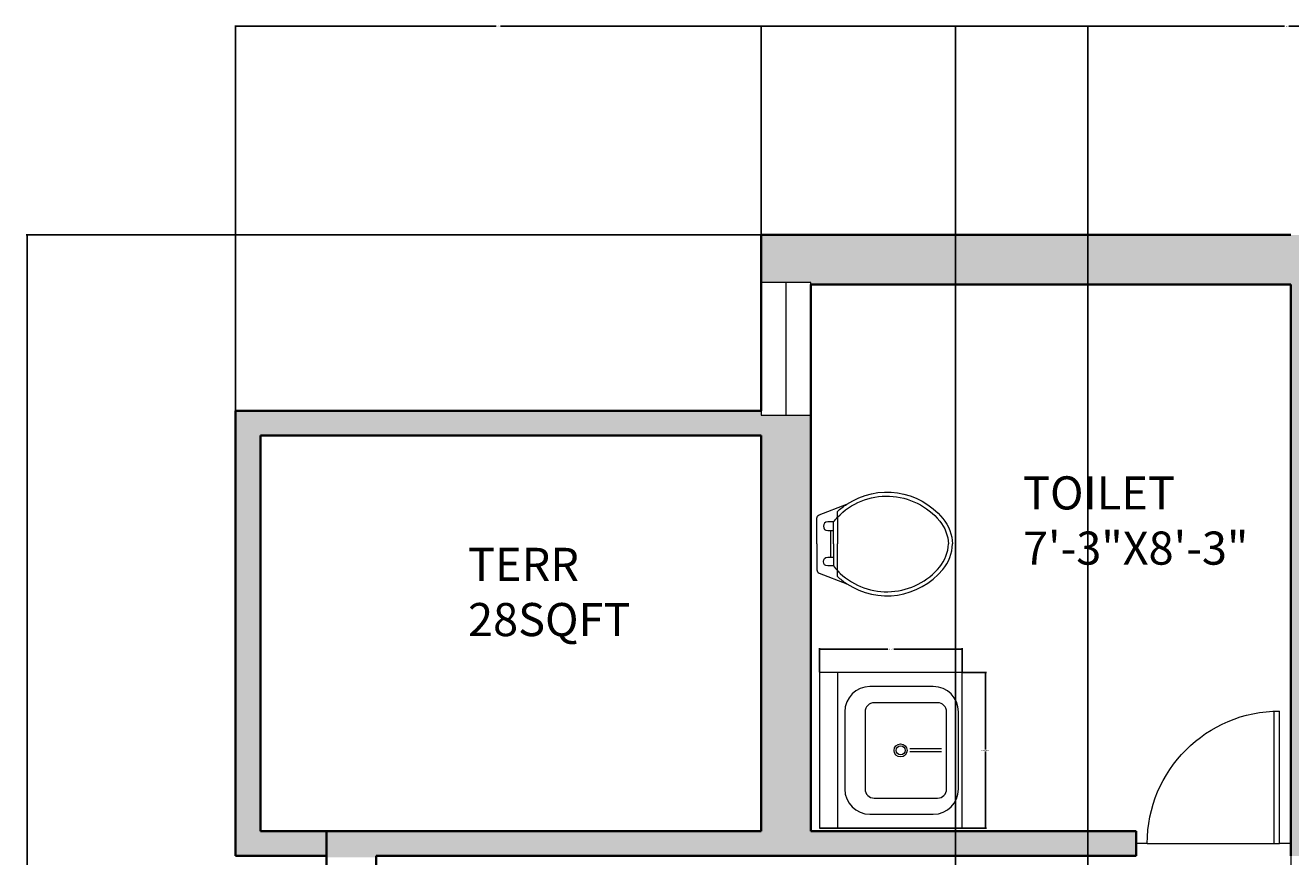
# Model space of a CAD drawing. Units: inches. Extents: x -36 to 442, y -676 to 151.
# Tile 6 of 8: x -36 to 193, y 1 to 151. Entities that reach past the tile are written whole.
import ezdxf

# ---------------------------------------------------------------- set-up
doc = ezdxf.new("R2010")
doc.units = ezdxf.units.IN
doc.header["$MEASUREMENT"] = 0
for name, color, linetype, lineweight in [('A-ANNO-DIMS', 2, 'Continuous', 18), ('A-AREA-IDEN', 7, 'Continuous', 18), ('A-DOOR', 4, 'Continuous', 18), ('A-FLOR-CASE', 32, 'Continuous', 18), ('A-FLOR-FIXT', 9, 'Continuous', 18), ('A-GLAZ', 4, 'Continuous', 13), ('A-WALL', 7, 'Continuous', 35), ('A-WALL-PATT', 8, 'Continuous', 13)]:
    doc.layers.add(name, color=color, linetype=linetype, lineweight=lineweight)
doc.styles.get("Standard").update_dxf_attribs({"font": 'arial.ttf'})
doc.dimstyles.get("Standard").update_dxf_attribs({"dimtxt": 0.18, "dimasz": 0.18, "dimexe": 0.18, "dimexo": 0.0625, "dimgap": 0.09, "dimtad": 0, "dimtih": 1, "dimtoh": 1, "dimdec": 0, "dimzin": 0, "dimdsep": 46, "dimlunit": 3, "dimtxsty": 'Standard', "dimcen": 0.09, "dimadec": 0, "dimazin": 0, "dimtfac": 1, "dimtdec": 0, "dimtofl": 0, "dimtmove": 0, "dimatfit": 3, "dimfxl": 1, "dimtolj": 1, "dimtzin": 0, "dimarcsym": 0})

# ---------------------------------------------------------------- blocks, each defined once
blk = doc.blocks.new('М14 600х655')
for p, q in [((-655, 600), (-655, 0)), ((-655, 600), (-655, 0)), ((-655, 0), (-655, 600)), ((0, 600), (-655, 600)), ((0, 0), (0, 600)), ((0, 525), (-655, 525)), ((-165.1, 494.1), (-489.9, 494.1)), ((-595.8, 388.1), (-595.8, 121.3)), ((-165.4, 408.4), (-490.2, 408.4)), ((-59.2, 121.3), (-59.2, 388.1)), ((-528.4, 370.1), (-528.4, 103.3)), ((-127.2, 103.3), (-127.2, 370.1)), ((-333.5, 87.1), (-333.5, 219.6)), ((-321.5, 87.1), (-321.5, 219.6)), ((-490.2, 65.1), (-165.4, 65.1)), ((-655, 0), (-655, 0)), ((-655, 0), (-655, 0)), ((-655, 0), (0, 0)), ((-655, 0), (0, 0)), ((-489.9, 15.4), (-165.1, 15.4))]:
    blk.add_line(p, q)
for radius in [27.6, 19.3]:
    blk.add_circle((-327.5, 258.9), radius)
for centre, radius, start, end in [((-489.9, 388.1), 105.9, 90, 180), ((-165.1, 388.1), 105.9, 0, 90), ((-490.2, 370.1), 38.2, 90, 180), ((-165.4, 370.1), 38.2, 0, 90), ((-489.9, 121.3), 105.9, 180, 270), ((-165.1, 121.3), 105.9, 270, 0), ((-490.2, 103.3), 38.2, 180, 270), ((-165.4, 103.3), 38.2, 270, 0)]:
    blk.add_arc(centre, radius, start, end)
blk = doc.blocks.new('DOOR-SWING-24IN')
for p, q in [((24, 26), (24, 28)), ((24, 26), (24, 2)), ((24, 3), (0, 3)), ((24, 2), (0, 2)), ((24, 0), (24, 2))]:
    blk.add_line(p, q)
blk.add_arc((24, 2), 24, 90, 180)
blk = doc.blocks.new('WC-PLAN')
for p, q in [((3.72, 14.23), (3.72, 15.26)), ((3.72, 14.23), (3.72, 9.39)), ((3.72, 4.56), (3.72, 9.39)), ((3.72, 3.52), (3.72, 4.56))]:
    blk.add_line(p, q)
for points in [[(5.41, 16.59, -0.383919), (22.82, 14.02, -0.163732), (24.59, 9.39, -0.359733)], [(0, 9.39), (0, 14.09, -0.31031), (0.4, 14.66), (5.41, 16.59, -0.209071)], [(3.72, 14.23, -0.448546), (22.25, 13.55, -0.162618), (23.85, 9.39, -0.470877)], [(3.72, 15.26, -0.040937), (5.41, 16.59, -0.163732)], [(2.98, 13.38, -0.022712), (3.72, 14.23, -0.162618)], [(2.98, 13.38), (1.95, 13.38, 1), (1.95, 11.81), (2.49, 11.81)], [(2.98, 9.39), (2.98, 13.38, -0.476108)], [(0, 9.39), (0, 4.7, 0.31031), (0.4, 4.12), (5.41, 2.19, 0.209071)], [(2.98, 9.39), (2.98, 5.4, 0.022712)], [(4.22, 4.06, 0.431639), (22.25, 5.24, 0.162618), (23.85, 9.39, 0.470877)], [(5.41, 2.19, 0.383919), (22.82, 4.77, 0.163732), (24.59, 9.39, 0.359733)], [(2.98, 5.4), (1.95, 5.4, -1), (1.95, 6.97), (2.49, 6.97)], [(2.98, 5.4, 0.022712), (3.72, 4.56, 0.162618)], [(3.72, 4.56, 0.014165), (4.22, 4.06, 0.162618)], [(3.72, 3.52, 0.040937), (5.41, 2.19, 0.163732)]]:
    blk.add_lwpolyline(points, format="xyb")
for points in [[(2.49, 11.81), (2.49, 6.97)], [(2.49, 11.81), (2.98, 11.81)], [(2.49, 6.97), (2.98, 6.97)]]:
    blk.add_lwpolyline(points)
blk = doc.blocks.new('*D27')
at = {"layer": 'A-ANNO-DIMS', "color": 0, "lineweight": -2, "transparency": 16777216}
for p, q in [((134, 34.23), (138.35, 34.23)), ((138.17, 34.05), (138.17, 20.31)), ((138.17, 6.2), (138.17, 19.94)), ((134, 6.02), (138.35, 6.02))]:
    blk.add_line(p, q, dxfattribs=at)
at = {"layer": 'A-ANNO-DIMS', "color": 0, "transparency": 16777216}
for points in [[(138.14, 34.05), (138.2, 34.05), (138.17, 34.23)], [(138.14, 6.2), (138.2, 6.2), (138.17, 6.02)]]:
    blk.add_solid(points, dxfattribs=at)
at = {"layer": 'Defpoints', "color": 0, "transparency": 16777216}
for p in [(133.94, 34.23), (138.17, 34.23), (133.94, 6.02)]:
    blk.add_point(p, dxfattribs=at)
at = {"layer": 'A-ANNO-DIMS', "color": 0, "transparency": 16777216, "insert": (138.17, 20.12), "char_height": 0.18, "attachment_point": 5}
blk.add_mtext('\\A1;BASIN 28 TYP.', dxfattribs=at)
blk = doc.blocks.new('*D28')
at = {"layer": 'A-ANNO-DIMS', "color": 0, "lineweight": -2, "transparency": 16777216}
for p, q in [((108.1, 34.29), (108.1, 38.64)), ((108.28, 38.46), (120.49, 38.46)), ((133.76, 38.46), (121.55, 38.46)), ((133.94, 34.29), (133.94, 38.64))]:
    blk.add_line(p, q, dxfattribs=at)
at = {"layer": 'A-ANNO-DIMS', "color": 0, "transparency": 16777216}
for points in [[(108.28, 38.49), (108.28, 38.43), (108.1, 38.46)], [(133.76, 38.49), (133.76, 38.43), (133.94, 38.46)]]:
    blk.add_solid(points, dxfattribs=at)
at = {"layer": 'Defpoints', "color": 0, "transparency": 16777216}
for p in [(108.1, 38.46), (108.1, 34.23), (133.94, 34.23)]:
    blk.add_point(p, dxfattribs=at)
at = {"layer": 'A-ANNO-DIMS', "color": 0, "transparency": 16777216, "insert": (121.02, 38.46), "char_height": 0.18, "attachment_point": 5}
blk.add_mtext('\\A1;26 TYP.', dxfattribs=at)
blk = doc.blocks.new('*D50')
at = {"layer": 'A-ANNO-DIMS', "color": 0, "lineweight": -2, "transparency": 16777216}
for p, q in [((97.44, 113.5), (-35.74, 113.5)), ((-35.56, 113.32), (-35.56, -262.07)), ((-35.56, -637.82), (-35.56, -262.43)), ((18.67, -638), (-35.74, -638))]:
    blk.add_line(p, q, dxfattribs=at)
at = {"layer": 'A-ANNO-DIMS', "color": 0, "transparency": 16777216}
for points in [[(-35.59, 113.32), (-35.53, 113.32), (-35.56, 113.5)], [(-35.59, -637.82), (-35.53, -637.82), (-35.56, -638)]]:
    blk.add_solid(points, dxfattribs=at)
at = {"layer": 'Defpoints', "color": 0, "transparency": 16777216}
for p in [(-35.56, 113.5), (97.5, 113.5), (18.74, -638)]:
    blk.add_point(p, dxfattribs=at)
at = {"layer": 'A-ANNO-DIMS', "color": 0, "transparency": 16777216, "insert": (-35.56, -262.25), "char_height": 0.18, "attachment_point": 5}
blk.add_mtext('\\A1;751.5', dxfattribs=at)
blk = doc.blocks.new('*D51')
at = {"layer": 'A-ANNO-DIMS', "color": 0, "lineweight": -2, "transparency": 16777216}
for p, q in [((2.24, 81.71), (2.24, 151.48)), ((97.5, 113.57), (97.5, 151.48)), ((2.42, 151.3), (49.47, 151.3)), ((97.32, 151.3), (50.26, 151.3))]:
    blk.add_line(p, q, dxfattribs=at)
at = {"layer": 'A-ANNO-DIMS', "color": 0, "transparency": 16777216}
for points in [[(2.42, 151.33), (2.42, 151.27), (2.24, 151.3)], [(97.32, 151.33), (97.32, 151.27), (97.5, 151.3)]]:
    blk.add_solid(points, dxfattribs=at)
at = {"layer": 'Defpoints', "color": 0, "transparency": 16777216}
for p in [(97.5, 151.3), (97.5, 113.5), (2.24, 81.65)]:
    blk.add_point(p, dxfattribs=at)
at = {"layer": 'A-ANNO-DIMS', "color": 0, "transparency": 16777216, "insert": (49.87, 151.3), "char_height": 0.18, "attachment_point": 5}
blk.add_mtext('\\A1;95.26', dxfattribs=at)
blk = doc.blocks.new('*D52')
at = {"layer": 'A-ANNO-DIMS', "color": 0, "lineweight": -2, "transparency": 16777216}
for p, q in [((97.5, 113.57), (97.5, 151.48)), ((288, 113.57), (288, 151.48)), ((97.68, 151.3), (192.36, 151.3)), ((287.82, 151.3), (193.14, 151.3))]:
    blk.add_line(p, q, dxfattribs=at)
at = {"layer": 'A-ANNO-DIMS', "color": 0, "transparency": 16777216}
for points in [[(97.68, 151.33), (97.68, 151.27), (97.5, 151.3)], [(287.82, 151.33), (287.82, 151.27), (288, 151.3)]]:
    blk.add_solid(points, dxfattribs=at)
at = {"layer": 'Defpoints', "color": 0, "transparency": 16777216}
for p in [(288, 151.3), (97.5, 113.5), (288, 113.5)]:
    blk.add_point(p, dxfattribs=at)
at = {"layer": 'A-ANNO-DIMS', "color": 0, "transparency": 16777216, "insert": (192.75, 151.3), "char_height": 0.18, "attachment_point": 5}
blk.add_mtext('\\A1;190.5', dxfattribs=at)
blk = doc.blocks.new('*D63')
at = {"layer": 'A-ANNO-DIMS', "color": 0, "lineweight": -2, "transparency": 16777216}
for p, q in [((132.74, -447.43), (132.74, 151.48)), ((156.74, -471.43), (156.74, 151.48)), ((132.92, 151.3), (144.51, 151.3)), ((156.56, 151.3), (144.96, 151.3))]:
    blk.add_line(p, q, dxfattribs=at)
at = {"layer": 'A-ANNO-DIMS', "color": 0, "transparency": 16777216}
for points in [[(132.92, 151.33), (132.92, 151.27), (132.74, 151.3)], [(156.56, 151.33), (156.56, 151.27), (156.74, 151.3)]]:
    blk.add_solid(points, dxfattribs=at)
at = {"layer": 'Defpoints', "color": 0, "transparency": 16777216}
for p in [(156.74, 151.3), (132.74, -447.5), (156.74, -471.5)]:
    blk.add_point(p, dxfattribs=at)
at = {"layer": 'A-ANNO-DIMS', "color": 0, "transparency": 16777216, "insert": (144.74, 151.3), "char_height": 0.18, "attachment_point": 5}
blk.add_mtext('\\A1;24', dxfattribs=at)

msp = doc.modelspace()

# ---------------------------------------------------------------- hatches: boundary and pattern name
at = {"layer": 'A-WALL-PATT'}
h = msp.add_hatch(color=256, dxfattribs=at)
h.dxf.hatch_style = 1
h.paths.add_polyline_path([(288, 113.503), (193.5, 113.503), (97.5, 113.503), (97.5, 104.864), (106.5, 104.864), (106.5, 104.503), (193.5, 104.503), (193.5, 5.503), (193.5, 1.003), (213.735, 1.003), (213.735, -135.497), (218.235, -135.497), (218.235, 1.003), (251, 1.003), (251, 3.253), (251, 5.503), (198, 5.503), (198, 104.503), (279, 104.503), (279, 104.209), (288, 104.209)])
h.paths.add_polyline_path([(378.735, 81.646), (362.235, 81.646), (288, 81.646), (288, 80.209), (279, 80.209), (279, 5.503), (279, 1.003), (353.235, 1.003), (353.235, 0.242), (362.235, 0.242), (362.235, 5.503), (288, 5.503), (288, 77.146), (362.235, 77.146), (374.235, 77.146), (374.235, 5.503), (362.235, 5.503), (362.235, 1.003), (374.235, 1.003), (378.735, 1.003), (378.735, 5.503), (378.735, 77.146)])
h.paths.add_polyline_path([(362.235, -35.758), (353.235, -35.758), (353.235, -196.997), (218.235, -196.997), (213.735, -196.997), (213.735, -205.997), (218.235, -205.997), (378.735, -205.997), (378.735, -205.779), (387.735, -205.779), (387.735, -202.472), (387.735, -196.997), (378.735, -196.997), (362.235, -196.997)])
h.paths.add_polyline_path([(218.235, -175.497), (215.985, -175.497), (213.735, -175.497), (213.735, -196.997), (218.235, -196.997)], flags=17)
h.paths.add_polyline_path([(158.235, -201.497), (98.235, -201.497), (98.235, -205.997), (158.235, -205.997)])
h.paths.add_polyline_path([(173.735, -130.997), (27.735, -130.997), (27.735, -35.267), (18.735, -35.267), (18.735, -138.68), (27.735, -138.68), (27.735, -135.497), (93.735, -135.497), (93.735, -201.497), (98.235, -201.497), (98.235, -135.497), (158.235, -135.497), (158.235, -173.497), (160.739, -173.497), (162.735, -173.497), (162.735, -135.497), (173.735, -135.497), (173.735, -133.017)])
h.paths.add_polyline_path([(98.235, -201.497), (93.735, -201.497), (93.735, -205.997), (98.235, -205.997)])
h.paths.add_polyline_path([(162.735, -201.497), (158.235, -201.497), (158.235, -205.997), (162.735, -205.997)])
h.paths.add_polyline_path([(63.735, -205.997), (63.735, -201.497), (27.735, -201.497), (27.735, -162.68), (18.735, -162.68), (18.735, -210.497), (63.735, -210.497)])
h.paths.add_polyline_path([(65.735, -203.604), (65.735, -201.497), (63.735, -201.497), (63.735, -205.997), (65.735, -205.997)])
h.paths.add_polyline_path([(165.5, 5.503), (106.5, 5.503), (106.5, 80.864), (97.5, 80.864), (97.5, 81.646), (6.735, 81.646), (2.235, 81.646), (2.235, 77.146), (2.235, 5.503), (2.235, 1.003), (6.735, 1.003), (18.735, 1.003), (18.735, 5.503), (6.735, 5.503), (6.735, 77.146), (97.5, 77.146), (97.5, 5.503), (18.735, 5.503), (18.735, 0.733), (27.735, 0.733), (27.735, 1.003), (165.5, 1.003), (165.5, 3.253)])
h.paths.add_polyline_path([(18.735, -201.497), (6.735, -201.497), (2.235, -201.497), (2.235, -210.497), (2.235, -354.497), (2.235, -363.497), (6.735, -363.497), (18.735, -363.497), (18.735, -358.997), (18.735, -354.497), (6.735, -354.497), (6.735, -210.497), (18.735, -210.497)])
h.paths.add_polyline_path([(63.735, -210.497), (54.735, -210.497), (54.735, -240.747), (63.735, -240.747)])
h.paths.add_polyline_path([(63.735, -336.747), (54.735, -336.747), (54.735, -354.497), (18.735, -354.497), (18.735, -358.997), (18.735, -363.497), (104.735, -363.497), (104.735, -361.247), (104.735, -358.997), (63.735, -358.997)])
h.paths.add_polyline_path([(27.735, -448.151), (18.735, -448.151), (18.735, -637.997), (72.735, -637.997), (72.735, -571.997), (183.235, -571.997), (183.235, -562.997), (57.197, -562.997), (51.735, -562.997), (51.735, -567.497), (57.197, -567.497), (63.735, -567.497), (63.735, -571.997), (63.735, -628.997), (27.735, -628.997), (27.735, -475.997), (27.735, -471.497)])
h.paths.add_polyline_path([(27.735, -363.497), (18.735, -363.497), (18.735, -412.151), (27.735, -412.151)])
h.paths.add_polyline_path([(161.235, -358.997), (132.735, -358.997), (132.735, -363.497), (156.735, -363.497), (156.735, -471.497), (51.735, -471.497), (51.735, -475.997), (63.735, -475.997), (63.735, -534.997), (65.985, -534.997), (68.235, -534.997), (68.235, -475.997), (161.235, -475.997)])
h.paths.add_polyline_path([(161.235, -511.997), (173.235, -511.997), (173.235, -502.997), (161.235, -502.997), (161.235, -475.997), (152.235, -475.997), (152.235, -534.997), (156.735, -534.997), (161.235, -534.997)], flags=17)
h.paths.add_polyline_path([(362.235, -502.997), (353.235, -502.997), (213.235, -502.997), (213.235, -507.497), (213.235, -511.997), (362.235, -511.997)])
h.paths.add_polyline_path([(242.235, -548.019), (233.235, -548.019), (233.235, -562.997), (223.235, -562.997), (223.235, -567.497), (223.235, -571.997), (242.235, -571.997)])
h.paths.add_polyline_path([(404.235, -502.997), (399.735, -502.997), (362.235, -502.997), (362.235, -511.997), (399.735, -511.997), (404.235, -511.997)])
h.paths.add_polyline_path([(362.235, -482.123), (353.235, -482.123), (353.235, -502.997), (362.235, -502.997)])
h.paths.add_polyline_path([(404.235, -295.997), (404.235, -286.997), (387.735, -286.997), (387.735, -295.997), (399.735, -295.997), (399.735, -502.997), (404.235, -502.997)])
h.paths.add_polyline_path([(362.235, -355.863), (353.235, -355.863), (353.235, -386.123), (362.235, -386.123)])
h.paths.add_polyline_path([(387.735, -286.997), (378.735, -286.997), (213.735, -286.997), (213.735, -295.997), (353.235, -295.997), (353.235, -295.863), (362.235, -295.863), (362.235, -295.997), (378.735, -295.997), (387.735, -295.997)])
h.paths.add_polyline_path([(387.735, -241.779), (378.735, -241.779), (378.735, -286.997), (387.735, -286.997)])
h.paths.add_polyline_path([(387.735, -175.497), (362.235, -175.497), (362.235, -184.497), (387.735, -184.497)], flags=17)
h.paths.add_polyline_path([(387.735, -184.497), (383.235, -184.497), (383.235, -192.497), (378.735, -192.497), (366.735, -192.497), (366.735, -184.497), (362.235, -184.497), (362.235, -196.997), (378.735, -196.997), (387.735, -196.997)], flags=17)
h.paths.add_polyline_path([(240.604, 40.967), (282.575, 40.967), (282.575, 63.356), (240.604, 63.356)], flags=25)

# ---------------------------------------------------------------- linework, layer by layer
at = {"layer": 'A-FLOR-CASE'}
msp.add_line((193.5, 1.003), (193.5, -58.997), dxfattribs=at)
at = {"layer": 'A-GLAZ'}
for p, q in [((97.5, 104.864), (97.5, 80.864)), ((106.5, 104.864), (97.5, 104.864)), ((102, 104.864), (102, 80.864)), ((106.5, 80.864), (106.5, 104.864)), ((97.5, 80.864), (106.5, 80.864))]:
    msp.add_line(p, q, dxfattribs=at)
at = {"layer": 'A-WALL'}
for p, q in [((97.5, 113.503), (193.5, 113.503)), ((97.5, 81.646), (97.5, 113.503)), ((106.5, 5.503), (106.5, 104.503)), ((106.5, 104.503), (193.5, 104.503)), ((193.5, 5.503), (193.5, 104.503)), ((2.235, 77.146), (2.235, 81.646)), ((2.235, 81.646), (6.735, 81.646)), ((6.735, 81.646), (97.5, 81.646)), ((2.235, 5.503), (2.235, 77.146)), ((6.735, 5.503), (6.735, 77.146)), ((6.735, 77.146), (97.5, 77.146)), ((97.5, 5.503), (97.5, 77.146)), ((2.235, 5.503), (2.235, 1.003)), ((18.735, 5.503), (6.735, 5.503)), ((18.735, 5.503), (18.735, -210.497)), ((18.735, 5.503), (97.5, 5.503)), ((106.5, 5.503), (165.5, 5.503)), ((165.5, 3.253), (165.5, 5.503)), ((193.5, 5.503), (193.5, 1.003)), ((165.5, 3.253), (165.5, 1.003)), ((2.235, 1.003), (6.735, 1.003)), ((18.735, 1.003), (6.735, 1.003)), ((27.735, 1.003), (165.5, 1.003)), ((27.735, 1.003), (27.735, -130.997))]:
    msp.add_line(p, q, dxfattribs=at)

# ---------------------------------------------------------------- block references
at = {"layer": 'A-DOOR', "extrusion": (0, 0, -1), "zscale": -1, "rotation": 270.0000000000005}
msp.add_blockref('DOOR-SWING-24IN', (-193.5, 27.253), dxfattribs=at)
at = {"layer": 'A-FLOR-FIXT'}
msp.add_blockref('WC-PLAN', (107.622, 48.132), dxfattribs=at)
at = {"layer": 'A-FLOR-FIXT', "xscale": 0.0430748895547816, "yscale": 0.0430748895547816, "zscale": 0.0430748895547816, "rotation": 90}
msp.add_blockref('М14 600х655', (133.941, 34.231), dxfattribs=at)

# ---------------------------------------------------------------- texts
at = {"layer": 'A-AREA-IDEN', "char_height": 6, "attachment_point": 1}
for s, insert in [('TOILET\\P7\'-3"X8\'-3"', (144.971, 69.773)), ('TERR\\P28SQFT', (44.373, 56.827))]:
    msp.add_mtext(s, dxfattribs=dict(at, insert=insert))

# ---------------------------------------------------------------- dimensions: what is measured, and where the dimension line sits
at = {"layer": 'A-ANNO-DIMS'}
for base, p1, p2, override, picture, middle in [((97.4998, 151.303), (2.2351, 81.6458), (97.4998, 113.503), {"dimdec": 2, "dimlfac": 1, "dimrnd": 0, "dimzin": 0, "dimdsep": 46, "dimlunit": 2}, '*D51', (49.8674, 151.303)), ((288, 151.303), (97.5, 113.503), (288, 113.503), {"dimdec": 1, "dimlfac": 1, "dimrnd": 0, "dimzin": 0, "dimdsep": 46, "dimlunit": 2}, '*D52', (192.75, 151.303)), ((156.735, 151.303), (132.735, -447.497), (156.735, -471.497), {"dimdec": 0, "dimlfac": 1, "dimrnd": 0, "dimzin": 0, "dimdsep": 46, "dimlunit": 2}, '*D63', (144.735, 151.303))]:
    dim = msp.add_linear_dim(base=base, p1=p1, p2=p2, dimstyle='Standard', override=override, dxfattribs=at)
    dim.commit()
    dim.dimension.update_dxf_attribs({"geometry": picture, "text_midpoint": middle})
dim = msp.add_linear_dim(base=(-35.565, 113.503), p1=(18.735, -637.997), p2=(97.5, 113.503), angle=90, dimstyle='Standard', override={"dimdec": 1, "dimlfac": 1, "dimrnd": 0, "dimzin": 0, "dimdsep": 46, "dimlunit": 2}, dxfattribs=at)
dim.commit()
dim.dimension.update_dxf_attribs({"geometry": '*D50', "text_midpoint": (-35.565, -262.247)})
for base, p1, p2, angle, text, picture, middle in [((108.096, 38.463), (133.941, 34.231), (108.096, 34.231), 180, '<> TYP.', '*D28', (121.018, 38.463)), ((138.173, 34.231), (133.941, 6.017), (133.941, 34.231), 90, 'BASIN <> TYP.', '*D27', (138.173, 20.124))]:
    dim = msp.add_linear_dim(base=base, p1=p1, p2=p2, angle=angle, text=text, dimstyle='Standard', override={"dimdec": 0, "dimlfac": 1, "dimrnd": 0, "dimzin": 0, "dimdsep": 46, "dimlunit": 2}, dxfattribs=at)
    dim.commit()
    dim.dimension.update_dxf_attribs({"geometry": picture, "text_midpoint": middle})

doc.saveas('drawing.dxf')
